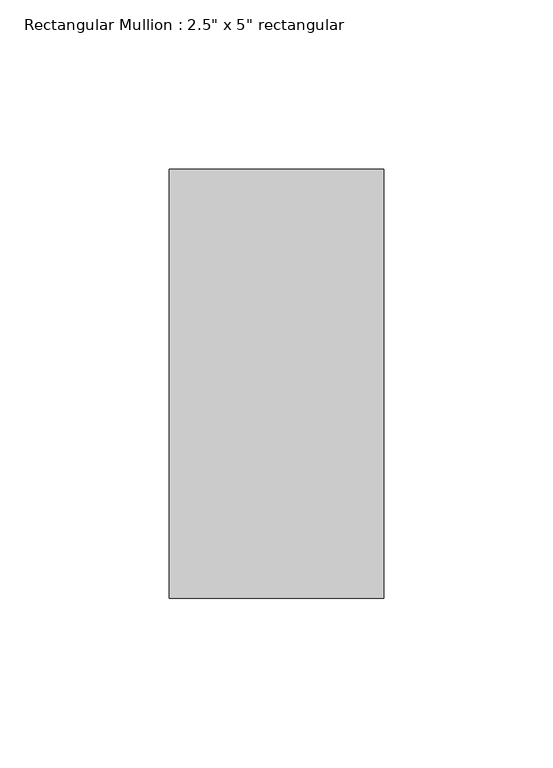
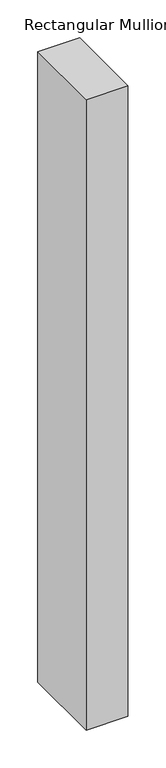
"""IFC4 building model written with IfcOpenShell, lengths in millimetres: member geometry."""

from ifc_helpers import new_model, si_unit, frame, origin, place, context, project, spatial, polyline, outline, extrude, source, transform, mapped, element, save


def member_852ada5c(model_context):
    return source(origin(), model_context, "Body", "SweptSolid", [
        extrude(outline(polyline([(31.75, 63.5), (31.75, -63.5), (-31.75, -63.5), (-31.75, 63.5), (31.75, 63.5)])), frame((0.0, 0.0, -1014.4047405), z_axis=(0.0, 0.0, 1.0), x_axis=(1.0, 0.0, 0.0)), (0.0, 0.0, 1.0), 1014.4047405),
    ])


if __name__ == "__main__":
    model = new_model("IFC4")
    model_context = context("Model", 3, world=origin())
    ifc_project = project(units=[si_unit("LENGTHUNIT", "METRE", prefix="MILLI")], contexts=[model_context])
    site = spatial("IfcSite", under=ifc_project)
    building = spatial("IfcBuilding", under=site)
    placement = place(None, origin())
    member_shape = member_852ada5c(model_context)
    element("IfcMember", 1, ObjectType="Rectangular Mullion : 2.5\" x 5\" rectangular", at=placement, inside=building, context=model_context, shape_type="MappedRepresentation", body=[
        mapped(member_shape, transform((0.0, 0.0, 0.0), x_axis=(1.0, 0.0, 0.0), y_axis=(0.0, 1.0, 0.0), z_axis=(0.0, 0.0, 1.0))),
    ])
    save(model, "model.ifc")

# Revit data of these elements
# Type "Rectangular Mullion : 2.5\" x 5\" rectangular"
#   built-in parameter 1007304 = 0.416667 (stored number, unit not read)
#   built-in parameter 1007301 = 0.104167 (stored number, unit not read)
#   built-in parameter 1007300 = 0.104167 (stored number, unit not read)
